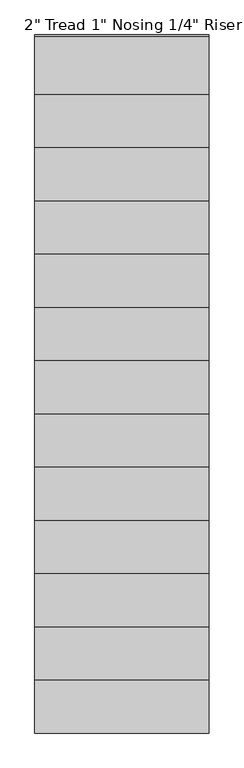
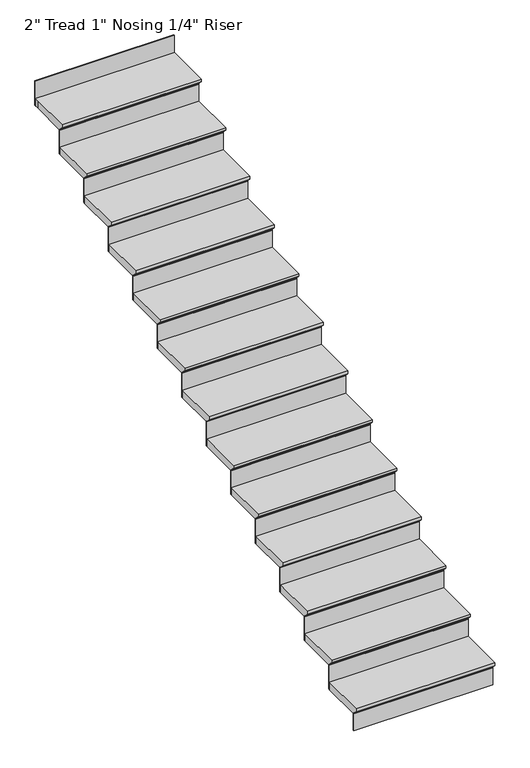
"""IFC4 building model written with IfcOpenShell, lengths in millimetres: stair flight geometry."""

from ifc_helpers import new_model, si_unit, origin, place, context, project, spatial, faceted_brep, source, transform, mapped, element, save


def stair_flight_a1121a25(model_context):
    return source(origin(), model_context, "Body", "Brep", [
        faceted_brep([(-2703.0415084, -23154.3851539, 40624.9005799), (-2703.0415084, -23154.3851539, 40643.9505799), (-3617.4415084, -23154.3851539, 40643.9505799), (-3617.4415084, -23154.3851539, 40624.9005799), (-2703.0415084, -23128.9851539, 40599.5005799), (-3617.4415084, -23128.9851539, 40599.5005799), (-2703.0415084, -22849.5851539, 40643.9505799), (-3617.4415084, -22849.5851539, 40643.9505799), (-3617.4415084, -23128.9851539, 40593.1505799), (-3617.4415084, -22849.5851539, 40593.1505799), (-2703.0415084, -22849.5851539, 40593.1505799), (-2703.0415084, -23128.9851539, 40593.1505799)], [[[0, 1, 2, 3]], [[4, 0, 3, 5]], [[2, 1, 6, 7]], [[8, 9, 10, 11]], [[2, 7, 9, 8, 5, 3]], [[8, 11, 4, 5]], [[6, 1, 0, 4, 11, 10]], [[7, 6, 10, 9]]]),
        faceted_brep([(-2703.0415084, -23128.9851539, 40593.1505799), (-2703.0415084, -23128.9851539, 40474.6172466), (-2703.0415084, -23122.6351539, 40474.6172466), (-2703.0415084, -23122.6351539, 40593.1505799), (-3617.4415084, -23128.9851539, 40593.1505799), (-3617.4415084, -23122.6351539, 40593.1505799), (-3617.4415084, -23122.6351539, 40474.6172466), (-3617.4415084, -23128.9851539, 40474.6172466)], [[[0, 1, 2, 3]], [[4, 5, 6, 7]], [[1, 0, 4, 7]], [[2, 1, 7, 6]], [[3, 2, 6, 5]], [[0, 3, 5, 4]]]),
        faceted_brep([(-2703.0415084, -22849.5851539, 40762.4839133), (-2703.0415084, -22849.5851539, 40593.1505799), (-2703.0415084, -22843.2351539, 40593.1505799), (-2703.0415084, -22843.2351539, 40762.4839133), (-3617.4415084, -22849.5851539, 40762.4839133), (-3617.4415084, -22843.2351539, 40762.4839133), (-3617.4415084, -22843.2351539, 40593.1505799), (-3617.4415084, -22849.5851539, 40593.1505799)], [[[0, 1, 2, 3]], [[4, 5, 6, 7]], [[1, 0, 4, 7]], [[2, 1, 7, 6]], [[3, 2, 6, 5]], [[0, 3, 5, 4]]]),
        faceted_brep([(-3617.4415084, -22874.9851539, 40813.2839133), (-2703.0415084, -22874.9851539, 40813.2839133), (-2703.0415084, -22570.1851539, 40813.2839133), (-3617.4415084, -22570.1851539, 40813.2839133), (-3617.4415084, -22849.5851539, 40762.4839133), (-3617.4415084, -22570.1851539, 40762.4839133), (-2703.0415084, -22570.1851539, 40762.4839133), (-2703.0415084, -22849.5851539, 40762.4839133), (-3617.4415084, -22849.5851539, 40768.8339133), (-3617.4415084, -22874.9851539, 40794.2339133), (-2703.0415084, -22849.5851539, 40768.8339133), (-2703.0415084, -22874.9851539, 40794.2339133)], [[[0, 1, 2, 3]], [[4, 5, 6, 7]], [[0, 3, 5, 4, 8, 9]], [[4, 7, 10, 8]], [[2, 1, 11, 10, 7, 6]], [[3, 2, 6, 5]], [[11, 1, 0, 9]], [[10, 11, 9, 8]]]),
        faceted_brep([(-2703.0415084, -22570.1851539, 40931.8172466), (-2703.0415084, -22570.1851539, 40762.4839133), (-2703.0415084, -22563.8351539, 40762.4839133), (-2703.0415084, -22563.8351539, 40931.8172466), (-3617.4415084, -22570.1851539, 40931.8172466), (-3617.4415084, -22563.8351539, 40931.8172466), (-3617.4415084, -22563.8351539, 40762.4839133), (-3617.4415084, -22570.1851539, 40762.4839133)], [[[0, 1, 2, 3]], [[4, 5, 6, 7]], [[1, 0, 4, 7]], [[2, 1, 7, 6]], [[3, 2, 6, 5]], [[0, 3, 5, 4]]]),
        faceted_brep([(-3617.4415084, -22595.5851539, 40982.6172466), (-2703.0415084, -22595.5851539, 40982.6172466), (-2703.0415084, -22290.7851539, 40982.6172466), (-3617.4415084, -22290.7851539, 40982.6172466), (-3617.4415084, -22570.1851539, 40931.8172466), (-3617.4415084, -22290.7851539, 40931.8172466), (-2703.0415084, -22290.7851539, 40931.8172466), (-2703.0415084, -22570.1851539, 40931.8172466), (-3617.4415084, -22570.1851539, 40938.1672466), (-3617.4415084, -22595.5851539, 40963.5672466), (-2703.0415084, -22570.1851539, 40938.1672466), (-2703.0415084, -22595.5851539, 40963.5672466)], [[[0, 1, 2, 3]], [[4, 5, 6, 7]], [[0, 3, 5, 4, 8, 9]], [[4, 7, 10, 8]], [[2, 1, 11, 10, 7, 6]], [[3, 2, 6, 5]], [[11, 1, 0, 9]], [[10, 11, 9, 8]]]),
        faceted_brep([(-2703.0415084, -22290.7851539, 41101.1505799), (-2703.0415084, -22290.7851539, 40931.8172466), (-2703.0415084, -22284.4351539, 40931.8172466), (-2703.0415084, -22284.4351539, 41101.1505799), (-3617.4415084, -22290.7851539, 41101.1505799), (-3617.4415084, -22284.4351539, 41101.1505799), (-3617.4415084, -22284.4351539, 40931.8172466), (-3617.4415084, -22290.7851539, 40931.8172466)], [[[0, 1, 2, 3]], [[4, 5, 6, 7]], [[1, 0, 4, 7]], [[2, 1, 7, 6]], [[3, 2, 6, 5]], [[0, 3, 5, 4]]]),
        faceted_brep([(-3617.4415084, -22316.1851539, 41151.9505799), (-2703.0415084, -22316.1851539, 41151.9505799), (-2703.0415084, -22011.3851539, 41151.9505799), (-3617.4415084, -22011.3851539, 41151.9505799), (-3617.4415084, -22290.7851539, 41101.1505799), (-3617.4415084, -22011.3851539, 41101.1505799), (-2703.0415084, -22011.3851539, 41101.1505799), (-2703.0415084, -22290.7851539, 41101.1505799), (-3617.4415084, -22290.7851539, 41107.5005799), (-3617.4415084, -22316.1851539, 41132.9005799), (-2703.0415084, -22290.7851539, 41107.5005799), (-2703.0415084, -22316.1851539, 41132.9005799)], [[[0, 1, 2, 3]], [[4, 5, 6, 7]], [[0, 3, 5, 4, 8, 9]], [[4, 7, 10, 8]], [[2, 1, 11, 10, 7, 6]], [[3, 2, 6, 5]], [[11, 1, 0, 9]], [[10, 11, 9, 8]]]),
        faceted_brep([(-2703.0415084, -22011.3851539, 41270.4839133), (-2703.0415084, -22011.3851539, 41101.1505799), (-2703.0415084, -22005.0351539, 41101.1505799), (-2703.0415084, -22005.0351539, 41270.4839133), (-3617.4415084, -22011.3851539, 41270.4839133), (-3617.4415084, -22005.0351539, 41270.4839133), (-3617.4415084, -22005.0351539, 41101.1505799), (-3617.4415084, -22011.3851539, 41101.1505799)], [[[0, 1, 2, 3]], [[4, 5, 6, 7]], [[1, 0, 4, 7]], [[2, 1, 7, 6]], [[3, 2, 6, 5]], [[0, 3, 5, 4]]]),
        faceted_brep([(-3617.4415084, -22036.7851539, 41321.2839133), (-2703.0415084, -22036.7851539, 41321.2839133), (-2703.0415084, -21731.9851539, 41321.2839133), (-3617.4415084, -21731.9851539, 41321.2839133), (-3617.4415084, -22011.3851539, 41270.4839133), (-3617.4415084, -21731.9851539, 41270.4839133), (-2703.0415084, -21731.9851539, 41270.4839133), (-2703.0415084, -22011.3851539, 41270.4839133), (-3617.4415084, -22011.3851539, 41276.8339133), (-3617.4415084, -22036.7851539, 41302.2339133), (-2703.0415084, -22011.3851539, 41276.8339133), (-2703.0415084, -22036.7851539, 41302.2339133)], [[[0, 1, 2, 3]], [[4, 5, 6, 7]], [[0, 3, 5, 4, 8, 9]], [[4, 7, 10, 8]], [[2, 1, 11, 10, 7, 6]], [[3, 2, 6, 5]], [[11, 1, 0, 9]], [[10, 11, 9, 8]]]),
        faceted_brep([(-2703.0415084, -21731.9851539, 41439.8172466), (-2703.0415084, -21731.9851539, 41270.4839133), (-2703.0415084, -21725.6351539, 41270.4839133), (-2703.0415084, -21725.6351539, 41439.8172466), (-3617.4415084, -21731.9851539, 41439.8172466), (-3617.4415084, -21725.6351539, 41439.8172466), (-3617.4415084, -21725.6351539, 41270.4839133), (-3617.4415084, -21731.9851539, 41270.4839133)], [[[0, 1, 2, 3]], [[4, 5, 6, 7]], [[1, 0, 4, 7]], [[2, 1, 7, 6]], [[3, 2, 6, 5]], [[0, 3, 5, 4]]]),
        faceted_brep([(-3617.4415084, -21757.3851539, 41490.6172466), (-2703.0415084, -21757.3851539, 41490.6172466), (-2703.0415084, -21452.5851539, 41490.6172466), (-3617.4415084, -21452.5851539, 41490.6172466), (-3617.4415084, -21731.9851539, 41439.8172466), (-3617.4415084, -21452.5851539, 41439.8172466), (-2703.0415084, -21452.5851539, 41439.8172466), (-2703.0415084, -21731.9851539, 41439.8172466), (-3617.4415084, -21731.9851539, 41446.1672466), (-3617.4415084, -21757.3851539, 41471.5672466), (-2703.0415084, -21731.9851539, 41446.1672466), (-2703.0415084, -21757.3851539, 41471.5672466)], [[[0, 1, 2, 3]], [[4, 5, 6, 7]], [[0, 3, 5, 4, 8, 9]], [[4, 7, 10, 8]], [[2, 1, 11, 10, 7, 6]], [[3, 2, 6, 5]], [[11, 1, 0, 9]], [[10, 11, 9, 8]]]),
        faceted_brep([(-2703.0415084, -21452.5851539, 41609.1505799), (-2703.0415084, -21452.5851539, 41439.8172466), (-2703.0415084, -21446.2351539, 41439.8172466), (-2703.0415084, -21446.2351539, 41609.1505799), (-3617.4415084, -21452.5851539, 41609.1505799), (-3617.4415084, -21446.2351539, 41609.1505799), (-3617.4415084, -21446.2351539, 41439.8172466), (-3617.4415084, -21452.5851539, 41439.8172466)], [[[0, 1, 2, 3]], [[4, 5, 6, 7]], [[1, 0, 4, 7]], [[2, 1, 7, 6]], [[3, 2, 6, 5]], [[0, 3, 5, 4]]]),
        faceted_brep([(-3617.4415084, -21477.9851539, 41659.9505799), (-2703.0415084, -21477.9851539, 41659.9505799), (-2703.0415084, -21173.1851539, 41659.9505799), (-3617.4415084, -21173.1851539, 41659.9505799), (-3617.4415084, -21452.5851539, 41609.1505799), (-3617.4415084, -21173.1851539, 41609.1505799), (-2703.0415084, -21173.1851539, 41609.1505799), (-2703.0415084, -21452.5851539, 41609.1505799), (-3617.4415084, -21452.5851539, 41615.5005799), (-3617.4415084, -21477.9851539, 41640.9005799), (-2703.0415084, -21452.5851539, 41615.5005799), (-2703.0415084, -21477.9851539, 41640.9005799)], [[[0, 1, 2, 3]], [[4, 5, 6, 7]], [[0, 3, 5, 4, 8, 9]], [[4, 7, 10, 8]], [[2, 1, 11, 10, 7, 6]], [[3, 2, 6, 5]], [[11, 1, 0, 9]], [[10, 11, 9, 8]]]),
        faceted_brep([(-2703.0415084, -21173.1851539, 41778.4839133), (-2703.0415084, -21173.1851539, 41609.1505799), (-2703.0415084, -21166.8351539, 41609.1505799), (-2703.0415084, -21166.8351539, 41778.4839133), (-3617.4415084, -21173.1851539, 41778.4839133), (-3617.4415084, -21166.8351539, 41778.4839133), (-3617.4415084, -21166.8351539, 41609.1505799), (-3617.4415084, -21173.1851539, 41609.1505799)], [[[0, 1, 2, 3]], [[4, 5, 6, 7]], [[1, 0, 4, 7]], [[2, 1, 7, 6]], [[3, 2, 6, 5]], [[0, 3, 5, 4]]]),
        faceted_brep([(-3617.4415084, -21198.5851539, 41829.2839133), (-2703.0415084, -21198.5851539, 41829.2839133), (-2703.0415084, -20893.7851539, 41829.2839133), (-3617.4415084, -20893.7851539, 41829.2839133), (-3617.4415084, -21173.1851539, 41778.4839133), (-3617.4415084, -20893.7851539, 41778.4839133), (-2703.0415084, -20893.7851539, 41778.4839133), (-2703.0415084, -21173.1851539, 41778.4839133), (-3617.4415084, -21173.1851539, 41784.8339133), (-3617.4415084, -21198.5851539, 41810.2339133), (-2703.0415084, -21173.1851539, 41784.8339133), (-2703.0415084, -21198.5851539, 41810.2339133)], [[[0, 1, 2, 3]], [[4, 5, 6, 7]], [[0, 3, 5, 4, 8, 9]], [[4, 7, 10, 8]], [[2, 1, 11, 10, 7, 6]], [[3, 2, 6, 5]], [[11, 1, 0, 9]], [[10, 11, 9, 8]]]),
        faceted_brep([(-2703.0415084, -20893.7851539, 41947.8172466), (-2703.0415084, -20893.7851539, 41778.4839133), (-2703.0415084, -20887.4351539, 41778.4839133), (-2703.0415084, -20887.4351539, 41947.8172466), (-3617.4415084, -20893.7851539, 41947.8172466), (-3617.4415084, -20887.4351539, 41947.8172466), (-3617.4415084, -20887.4351539, 41778.4839133), (-3617.4415084, -20893.7851539, 41778.4839133)], [[[0, 1, 2, 3]], [[4, 5, 6, 7]], [[1, 0, 4, 7]], [[2, 1, 7, 6]], [[3, 2, 6, 5]], [[0, 3, 5, 4]]]),
        faceted_brep([(-3617.4415084, -20919.1851539, 41998.6172466), (-2703.0415084, -20919.1851539, 41998.6172466), (-2703.0415084, -20614.3851539, 41998.6172466), (-3617.4415084, -20614.3851539, 41998.6172466), (-3617.4415084, -20893.7851539, 41947.8172466), (-3617.4415084, -20614.3851539, 41947.8172466), (-2703.0415084, -20614.3851539, 41947.8172466), (-2703.0415084, -20893.7851539, 41947.8172466), (-3617.4415084, -20893.7851539, 41954.1672466), (-3617.4415084, -20919.1851539, 41979.5672466), (-2703.0415084, -20893.7851539, 41954.1672466), (-2703.0415084, -20919.1851539, 41979.5672466)], [[[0, 1, 2, 3]], [[4, 5, 6, 7]], [[0, 3, 5, 4, 8, 9]], [[4, 7, 10, 8]], [[2, 1, 11, 10, 7, 6]], [[3, 2, 6, 5]], [[11, 1, 0, 9]], [[10, 11, 9, 8]]]),
        faceted_brep([(-2703.0415084, -20614.3851539, 42117.1505799), (-2703.0415084, -20614.3851539, 41947.8172466), (-2703.0415084, -20608.0351539, 41947.8172466), (-2703.0415084, -20608.0351539, 42117.1505799), (-3617.4415084, -20614.3851539, 42117.1505799), (-3617.4415084, -20608.0351539, 42117.1505799), (-3617.4415084, -20608.0351539, 41947.8172466), (-3617.4415084, -20614.3851539, 41947.8172466)], [[[0, 1, 2, 3]], [[4, 5, 6, 7]], [[1, 0, 4, 7]], [[2, 1, 7, 6]], [[3, 2, 6, 5]], [[0, 3, 5, 4]]]),
        faceted_brep([(-3617.4415084, -20639.7851539, 42167.9505799), (-2703.0415084, -20639.7851539, 42167.9505799), (-2703.0415084, -20334.9851539, 42167.9505799), (-3617.4415084, -20334.9851539, 42167.9505799), (-3617.4415084, -20614.3851539, 42117.1505799), (-3617.4415084, -20334.9851539, 42117.1505799), (-2703.0415084, -20334.9851539, 42117.1505799), (-2703.0415084, -20614.3851539, 42117.1505799), (-3617.4415084, -20614.3851539, 42123.5005799), (-3617.4415084, -20639.7851539, 42148.9005799), (-2703.0415084, -20614.3851539, 42123.5005799), (-2703.0415084, -20639.7851539, 42148.9005799)], [[[0, 1, 2, 3]], [[4, 5, 6, 7]], [[0, 3, 5, 4, 8, 9]], [[4, 7, 10, 8]], [[2, 1, 11, 10, 7, 6]], [[3, 2, 6, 5]], [[11, 1, 0, 9]], [[10, 11, 9, 8]]]),
        faceted_brep([(-2703.0415084, -20334.9851539, 42286.4839133), (-2703.0415084, -20334.9851539, 42117.1505799), (-2703.0415084, -20328.6351539, 42117.1505799), (-2703.0415084, -20328.6351539, 42286.4839133), (-3617.4415084, -20334.9851539, 42286.4839133), (-3617.4415084, -20328.6351539, 42286.4839133), (-3617.4415084, -20328.6351539, 42117.1505799), (-3617.4415084, -20334.9851539, 42117.1505799)], [[[0, 1, 2, 3]], [[4, 5, 6, 7]], [[1, 0, 4, 7]], [[2, 1, 7, 6]], [[3, 2, 6, 5]], [[0, 3, 5, 4]]]),
        faceted_brep([(-3617.4415084, -20360.3851539, 42337.2839133), (-2703.0415084, -20360.3851539, 42337.2839133), (-2703.0415084, -20055.5851539, 42337.2839133), (-3617.4415084, -20055.5851539, 42337.2839133), (-3617.4415084, -20334.9851539, 42286.4839133), (-3617.4415084, -20055.5851539, 42286.4839133), (-2703.0415084, -20055.5851539, 42286.4839133), (-2703.0415084, -20334.9851539, 42286.4839133), (-3617.4415084, -20334.9851539, 42292.8339133), (-3617.4415084, -20360.3851539, 42318.2339133), (-2703.0415084, -20334.9851539, 42292.8339133), (-2703.0415084, -20360.3851539, 42318.2339133)], [[[0, 1, 2, 3]], [[4, 5, 6, 7]], [[0, 3, 5, 4, 8, 9]], [[4, 7, 10, 8]], [[2, 1, 11, 10, 7, 6]], [[3, 2, 6, 5]], [[11, 1, 0, 9]], [[10, 11, 9, 8]]]),
        faceted_brep([(-2703.0415084, -20055.5851539, 42455.8172466), (-2703.0415084, -20055.5851539, 42286.4839133), (-2703.0415084, -20049.2351539, 42286.4839133), (-2703.0415084, -20049.2351539, 42455.8172466), (-3617.4415084, -20055.5851539, 42455.8172466), (-3617.4415084, -20049.2351539, 42455.8172466), (-3617.4415084, -20049.2351539, 42286.4839133), (-3617.4415084, -20055.5851539, 42286.4839133)], [[[0, 1, 2, 3]], [[4, 5, 6, 7]], [[1, 0, 4, 7]], [[2, 1, 7, 6]], [[3, 2, 6, 5]], [[0, 3, 5, 4]]]),
        faceted_brep([(-3617.4415084, -20080.9851539, 42506.6172466), (-2703.0415084, -20080.9851539, 42506.6172466), (-2703.0415084, -19776.1851539, 42506.6172466), (-3617.4415084, -19776.1851539, 42506.6172466), (-3617.4415084, -20055.5851539, 42455.8172466), (-3617.4415084, -19776.1851539, 42455.8172466), (-2703.0415084, -19776.1851539, 42455.8172466), (-2703.0415084, -20055.5851539, 42455.8172466), (-3617.4415084, -20055.5851539, 42462.1672466), (-3617.4415084, -20080.9851539, 42487.5672466), (-2703.0415084, -20055.5851539, 42462.1672466), (-2703.0415084, -20080.9851539, 42487.5672466)], [[[0, 1, 2, 3]], [[4, 5, 6, 7]], [[0, 3, 5, 4, 8, 9]], [[4, 7, 10, 8]], [[2, 1, 11, 10, 7, 6]], [[3, 2, 6, 5]], [[11, 1, 0, 9]], [[10, 11, 9, 8]]]),
        faceted_brep([(-2703.0415084, -19496.7851539, 42794.4839133), (-2703.0415084, -19496.7851539, 42625.1505799), (-2703.0415084, -19490.4351539, 42625.1505799), (-2703.0415084, -19490.4351539, 42794.4839133), (-3617.4415084, -19496.7851539, 42794.4839133), (-3617.4415084, -19490.4351539, 42794.4839133), (-3617.4415084, -19490.4351539, 42625.1505799), (-3617.4415084, -19496.7851539, 42625.1505799)], [[[0, 1, 2, 3]], [[4, 5, 6, 7]], [[1, 0, 4, 7]], [[2, 1, 7, 6]], [[3, 2, 6, 5]], [[0, 3, 5, 4]]]),
        faceted_brep([(-2703.0415084, -19776.1851539, 42625.1505799), (-2703.0415084, -19776.1851539, 42455.8172466), (-2703.0415084, -19769.8351539, 42455.8172466), (-2703.0415084, -19769.8351539, 42625.1505799), (-3617.4415084, -19776.1851539, 42625.1505799), (-3617.4415084, -19769.8351539, 42625.1505799), (-3617.4415084, -19769.8351539, 42455.8172466), (-3617.4415084, -19776.1851539, 42455.8172466)], [[[0, 1, 2, 3]], [[4, 5, 6, 7]], [[1, 0, 4, 7]], [[2, 1, 7, 6]], [[3, 2, 6, 5]], [[0, 3, 5, 4]]]),
        faceted_brep([(-3617.4415084, -19496.7851539, 42675.9505799), (-3617.4415084, -19522.1851539, 42675.9505799), (-3617.4415084, -19801.5851539, 42675.9505799), (-2703.0415084, -19801.5851539, 42675.9505799), (-2703.0415084, -19496.7851539, 42675.9505799), (-3617.4415084, -19522.1851539, 42625.1505799), (-3617.4415084, -19496.7851539, 42625.1505799), (-2703.0415084, -19496.7851539, 42625.1505799), (-2703.0415084, -19776.1851539, 42625.1505799), (-3617.4415084, -19776.1851539, 42625.1505799), (-3617.4415084, -19776.1851539, 42631.5005799), (-3617.4415084, -19801.5851539, 42656.9005799), (-2703.0415084, -19776.1851539, 42631.5005799), (-2703.0415084, -19801.5851539, 42656.9005799)], [[[0, 1, 2, 3, 4]], [[5, 6, 7, 8, 9]], [[1, 0, 6, 5]], [[2, 1, 5, 9, 10, 11]], [[9, 8, 12, 10]], [[4, 3, 13, 12, 8, 7]], [[0, 4, 7, 6]], [[13, 3, 2, 11]], [[12, 13, 11, 10]]]),
    ])


if __name__ == "__main__":
    model = new_model("IFC4")
    model_context = context("Model", 3, world=origin())
    ifc_project = project(units=[si_unit("LENGTHUNIT", "METRE", prefix="MILLI")], contexts=[model_context])
    site = spatial("IfcSite", under=ifc_project)
    building = spatial("IfcBuilding", under=site)
    placement = place(None, origin())
    stair_flight_shape = stair_flight_a1121a25(model_context)
    element("IfcStairFlight", 1, ObjectType="2\" Tread 1\" Nosing 1/4\" Riser", at=placement, inside=building, context=model_context, shape_type="MappedRepresentation", body=[
        mapped(stair_flight_shape, transform((0.0, 0.0, 0.0), x_axis=(1.0, 0.0, 0.0), y_axis=(0.0, 1.0, 0.0), z_axis=(0.0, 0.0, 1.0))),
    ])
    save(model, "model.ifc")
